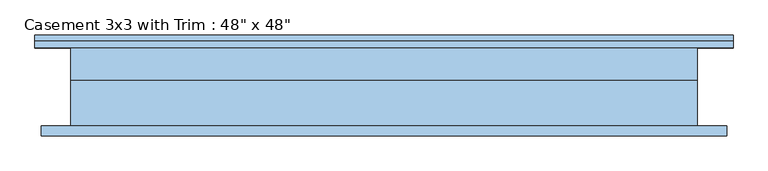
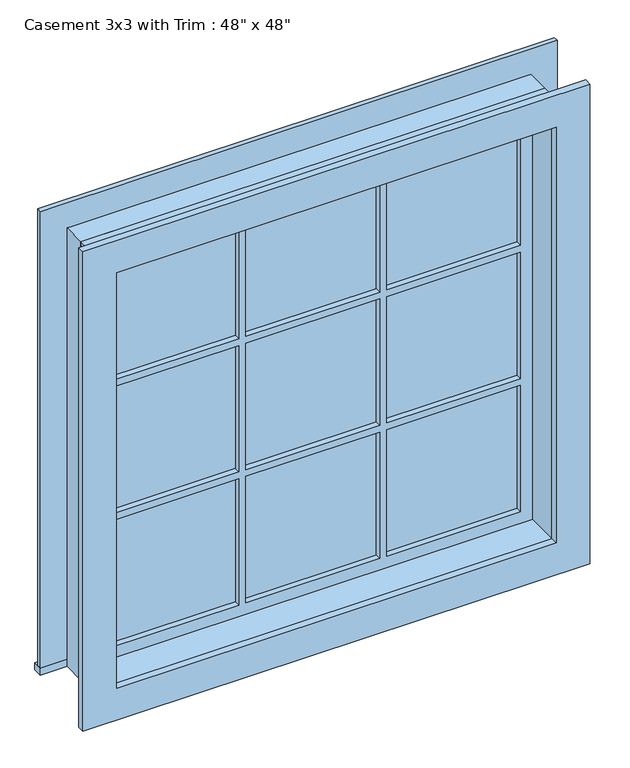
"""IFC4 building model written with IfcOpenShell, lengths in millimetres: window geometry."""

from ifc_helpers import new_model, si_unit, frame, origin, place, context, project, spatial, polyline, outline, extrude, source, transform, mapped, element, save


def window_7e6ae3b0(model_context):
    return source(origin(), model_context, "Body", "SweptSolid", [
        extrude(outline(polyline([(-679.45, 101.6), (679.45, 101.6), (679.45, 76.2), (-679.45, 76.2), (-679.45, 101.6)])), frame((0.0, 0.0, 914.4), z_axis=(0.0, 0.0, 1.0), x_axis=(1.0, 0.0, 0.0)), (0.0, 0.0, 1.0), 19.05),
        extrude(outline(polyline([(2114.55, -590.55), (2114.55, 590.55), (933.45, 590.55), (933.45, 679.45), (2203.45, 679.45), (2203.45, -679.45), (933.45, -679.45), (933.45, -590.55), (2114.55, -590.55)])), frame((0.0, 76.2, 0.0), z_axis=(0.0, 1.0, 0.0), x_axis=(0.0, 0.0, 1.0)), (0.0, 0.0, 1.0), 12.7),
        extrude(outline(polyline([(194.7333333, 41.275), (546.1, 41.275), (546.1, 28.575), (194.7333333, 28.575), (194.7333333, 41.275)])), frame((0.0, 0.0, 1718.7333333), z_axis=(0.0, 0.0, 1.0), x_axis=(1.0, 0.0, 0.0)), (0.0, 0.0, 1.0), 351.3666667),
        extrude(outline(polyline([(-175.6833333, 41.275), (175.6833333, 41.275), (175.6833333, 28.575), (-175.6833333, 28.575), (-175.6833333, 41.275)])), frame((0.0, 0.0, 1718.7333333), z_axis=(0.0, 0.0, 1.0), x_axis=(1.0, 0.0, 0.0)), (0.0, 0.0, 1.0), 351.3666667),
        extrude(outline(polyline([(-546.1, 41.275), (-194.7333333, 41.275), (-194.7333333, 28.575), (-546.1, 28.575), (-546.1, 41.275)])), frame((0.0, 0.0, 1718.7333333), z_axis=(0.0, 0.0, 1.0), x_axis=(1.0, 0.0, 0.0)), (0.0, 0.0, 1.0), 351.3666667),
        extrude(outline(polyline([(-546.1, 41.275), (-194.7333333, 41.275), (-194.7333333, 28.575), (-546.1, 28.575), (-546.1, 41.275)])), frame((0.0, 0.0, 1348.3166667), z_axis=(0.0, 0.0, 1.0), x_axis=(1.0, 0.0, 0.0)), (0.0, 0.0, 1.0), 351.3666667),
        extrude(outline(polyline([(-175.6833333, 41.275), (175.6833333, 41.275), (175.6833333, 28.575), (-175.6833333, 28.575), (-175.6833333, 41.275)])), frame((0.0, 0.0, 1348.3166667), z_axis=(0.0, 0.0, 1.0), x_axis=(1.0, 0.0, 0.0)), (0.0, 0.0, 1.0), 351.3666667),
        extrude(outline(polyline([(194.7333333, 41.275), (546.1, 41.275), (546.1, 28.575), (194.7333333, 28.575), (194.7333333, 41.275)])), frame((0.0, 0.0, 1348.3166667), z_axis=(0.0, 0.0, 1.0), x_axis=(1.0, 0.0, 0.0)), (0.0, 0.0, 1.0), 351.3666667),
        extrude(outline(polyline([(194.7333333, 41.275), (546.1, 41.275), (546.1, 28.575), (194.7333333, 28.575), (194.7333333, 41.275)])), frame((0.0, 0.0, 977.9), z_axis=(0.0, 0.0, 1.0), x_axis=(1.0, 0.0, 0.0)), (0.0, 0.0, 1.0), 351.3666667),
        extrude(outline(polyline([(-175.6833333, 41.275), (175.6833333, 41.275), (175.6833333, 28.575), (-175.6833333, 28.575), (-175.6833333, 41.275)])), frame((0.0, 0.0, 977.9), z_axis=(0.0, 0.0, 1.0), x_axis=(1.0, 0.0, 0.0)), (0.0, 0.0, 1.0), 351.3666667),
        extrude(outline(polyline([(-546.1, 41.275), (-194.7333333, 41.275), (-194.7333333, 28.575), (-546.1, 28.575), (-546.1, 41.275)])), frame((0.0, 0.0, 977.9), z_axis=(0.0, 0.0, 1.0), x_axis=(1.0, 0.0, 0.0)), (0.0, 0.0, 1.0), 351.3666667),
        extrude(outline(polyline([(2190.75, 666.75), (2190.75, -666.75), (857.25, -666.75), (857.25, 666.75), (2190.75, 666.75)]), holes=[polyline([(2101.85, 577.85), (946.15, 577.85), (946.15, -577.85), (2101.85, -577.85), (2101.85, 577.85)])]), frame((0.0, -95.25, 0.0), z_axis=(0.0, 1.0, 0.0), x_axis=(0.0, 0.0, 1.0)), (0.0, 0.0, 1.0), 19.05),
        extrude(outline(polyline([(2114.55, -590.55), (933.45, -590.55), (933.45, 590.55), (2114.55, 590.55), (2114.55, -590.55)]), holes=[polyline([(2070.1, -194.7333333), (1718.7333333, -194.7333333), (1718.7333333, -546.1), (2070.1, -546.1), (2070.1, -194.7333333)]), polyline([(1699.6833333, -194.7333333), (1348.3166667, -194.7333333), (1348.3166667, -546.1), (1699.6833333, -546.1), (1699.6833333, -194.7333333)]), polyline([(1329.2666667, -194.7333333), (977.9, -194.7333333), (977.9, -546.1), (1329.2666667, -546.1), (1329.2666667, -194.7333333)]), polyline([(2070.1, 175.6833333), (1718.7333333, 175.6833333), (1718.7333333, -175.6833333), (2070.1, -175.6833333), (2070.1, 175.6833333)]), polyline([(1699.6833333, 175.6833333), (1348.3166667, 175.6833333), (1348.3166667, -175.6833333), (1699.6833333, -175.6833333), (1699.6833333, 175.6833333)]), polyline([(1329.2666667, 175.6833333), (977.9, 175.6833333), (977.9, -175.6833333), (1329.2666667, -175.6833333), (1329.2666667, 175.6833333)]), polyline([(2070.1, 546.1), (1718.7333333, 546.1), (1718.7333333, 194.7333333), (2070.1, 194.7333333), (2070.1, 546.1)]), polyline([(1699.6833333, 546.1), (1348.3166667, 546.1), (1348.3166667, 194.7333333), (1699.6833333, 194.7333333), (1699.6833333, 546.1)]), polyline([(1329.2666667, 546.1), (977.9, 546.1), (977.9, 194.7333333), (1329.2666667, 194.7333333), (1329.2666667, 546.1)])]), frame((0.0, 12.7, 0.0), z_axis=(0.0, 1.0, 0.0), x_axis=(0.0, 0.0, 1.0)), (0.0, 0.0, 1.0), 44.45),
        extrude(outline(polyline([(2133.6, -609.6), (914.4, -609.6), (914.4, 609.6), (2133.6, 609.6), (2133.6, -609.6)]), holes=[polyline([(2101.85, -577.85), (2101.85, 577.85), (946.15, 577.85), (946.15, -577.85), (2101.85, -577.85)])]), frame((0.0, -76.2, 0.0), z_axis=(0.0, 1.0, 0.0), x_axis=(0.0, 0.0, 1.0)), (0.0, 0.0, 1.0), 88.9),
        extrude(outline(polyline([(2133.6, 609.6), (2133.6, -609.6), (914.4, -609.6), (914.4, 609.6), (2133.6, 609.6)]), holes=[polyline([(2114.55, 590.55), (933.45, 590.55), (933.45, -590.55), (2114.55, -590.55), (2114.55, 590.55)])]), frame((0.0, 12.7, 0.0), z_axis=(0.0, 1.0, 0.0), x_axis=(0.0, 0.0, 1.0)), (0.0, 0.0, 1.0), 63.5),
    ])


if __name__ == "__main__":
    model = new_model("IFC4")
    model_context = context("Model", 3, world=origin())
    ifc_project = project(units=[si_unit("LENGTHUNIT", "METRE", prefix="MILLI")], contexts=[model_context])
    site = spatial("IfcSite", under=ifc_project)
    building = spatial("IfcBuilding", under=site)
    placement = place(None, origin())
    window_shape = window_7e6ae3b0(model_context)
    element("IfcWindow", 1, ObjectType="Casement 3x3 with Trim : 48\" x 48\"", at=placement, inside=building, context=model_context, shape_type="MappedRepresentation", body=[
        mapped(window_shape, transform((0.0, 0.0, 0.0), x_axis=(1.0, 0.0, 0.0), y_axis=(0.0, 1.0, 0.0), z_axis=(0.0, 0.0, 1.0))),
    ])
    save(model, "model.ifc")

# Revit data of these elements
# Type "Casement 3x3 with Trim : 48\" x 48\""
#   Type Mark = "10"
#   Construction Type Id = "GSP4R"
#   Assembly Code = "B2020100"
#   Analytic Construction = "1/8 in Pilkington single glazing"
#   Visual Light Transmittance = 0.9
#   Solar Heat Gain Coefficient = 0.78
#   Heat Transfer Coefficient (U) = 0.6496 BTU/(h·ft²·°F)
#   Height = 4' - 0"
#   Default Sill Height = 3' - 0"
#   Trim Projection - Ext. = 0' - 0 1/2"
#   Trim Projection - Int. = 0' - 0 3/4"
#   Trim Width - Exterior = 0' - 3 1/2"
#   Trim Width - Interior = 0' - 3 1/2"
#   Width = 4' - 0"
#   Window Inset = 0' - 0 3/4"
#   Define Thermal Properties by = 1
#   Glass Pane Material = Glass
#   Sash Material = Sash
#   Trim Exterior Material = Trim
#   Trim Interior Material = Trim
#   Wall Closure = (empty or 0)
# Element 1 (IfcWindow, "Casement 3x3 with Trim : 48\" x 48\"")
#   Materials on its faces: "Sash", "Glass", "Trim"
# Materials
#   "Glass": class "Glass", colour RGB 0 128 192, transparency 0.75, Description = "Soda Lime Glass", Cost = 0
#   "Sash": class "Wood", colour RGB 224 178 126, transparency 0
#   "Trim": class "Wood", colour RGB 224 178 126, transparency 0
